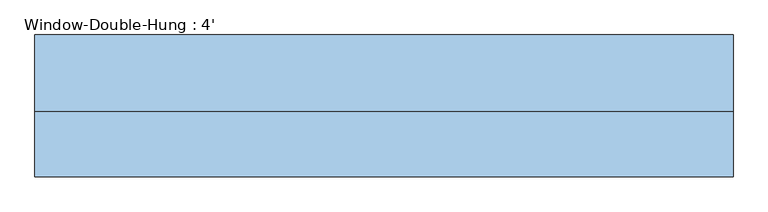
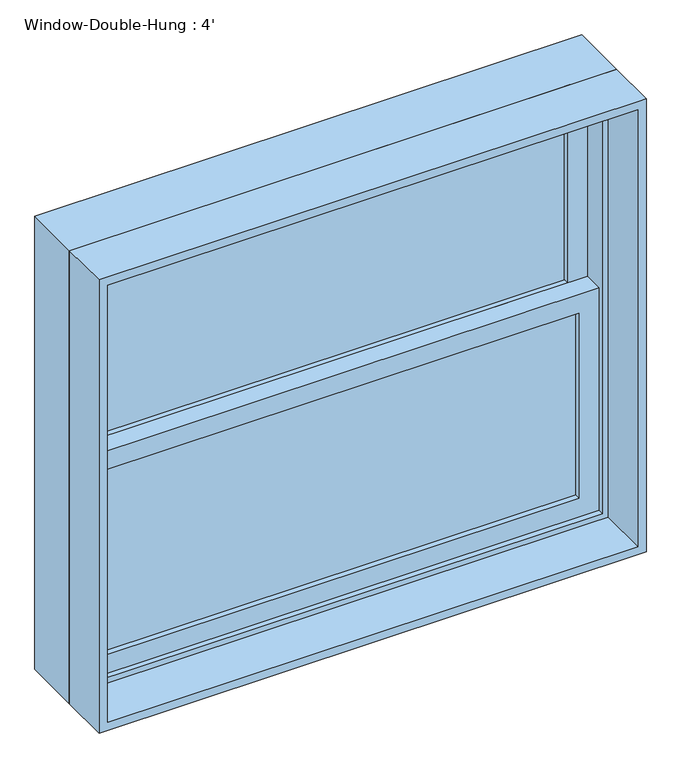
"""IFC4 building model written with IfcOpenShell, lengths in millimetres: window geometry, Window-Double-Hung : 4'."""

from ifc_helpers import new_model, si_unit, frame, origin, place, context, project, spatial, polyline, outline, extrude, source, transform, mapped, element, save


def window_double_hung_4_eadb0177(model_context):
    return source(origin(), model_context, "Body", "SweptSolid", [
        extrude(outline(polyline([(533.4, 44.45), (533.4, 38.1), (-533.4, 38.1), (-533.4, 44.45), (533.4, 44.45)])), frame((0.0, 0.0, 990.6), z_axis=(0.0, 0.0, 1.0), x_axis=(1.0, 0.0, 0.0)), (0.0, 0.0, 1.0), 434.975),
        extrude(outline(polyline([(-533.4, 31.75), (533.4, 31.75), (533.4, 25.4), (-533.4, 25.4), (-533.4, 31.75)])), frame((0.0, 0.0, 990.6), z_axis=(0.0, 0.0, 1.0), x_axis=(1.0, 0.0, 0.0)), (0.0, 0.0, 1.0), 434.975),
        extrude(outline(polyline([(533.4, 88.9), (533.4, 82.55), (-533.4, 82.55), (-533.4, 88.9), (533.4, 88.9)])), frame((0.0, 0.0, 1470.025), z_axis=(0.0, 0.0, 1.0), x_axis=(1.0, 0.0, 0.0)), (0.0, 0.0, 1.0), 434.975),
        extrude(outline(polyline([(-533.4, 76.2), (533.4, 76.2), (533.4, 69.85), (-533.4, 69.85), (-533.4, 76.2)])), frame((0.0, 0.0, 1470.025), z_axis=(0.0, 0.0, 1.0), x_axis=(1.0, 0.0, 0.0)), (0.0, 0.0, 1.0), 434.975),
        extrude(outline(polyline([(1470.025, -577.85), (946.15, -577.85), (946.15, 577.85), (1470.025, 577.85), (1470.025, -577.85)]), holes=[polyline([(1425.575, 533.4), (990.6, 533.4), (990.6, -533.4), (1425.575, -533.4), (1425.575, 533.4)])]), frame((0.0, 12.7, 0.0), z_axis=(0.0, 1.0, 0.0), x_axis=(0.0, 0.0, 1.0)), (0.0, 0.0, 1.0), 44.45),
        extrude(outline(polyline([(1949.45, -577.85), (1425.575, -577.85), (1425.575, 577.85), (1949.45, 577.85), (1949.45, -577.85)]), holes=[polyline([(1905.0, 533.4), (1470.025, 533.4), (1470.025, -533.4), (1905.0, -533.4), (1905.0, 533.4)])]), frame((0.0, 57.15, 0.0), z_axis=(0.0, 1.0, 0.0), x_axis=(0.0, 0.0, 1.0)), (0.0, 0.0, 1.0), 44.45),
        extrude(outline(polyline([(1981.2, -609.6), (914.4, -609.6), (914.4, 609.6), (1981.2, 609.6), (1981.2, -609.6)]), holes=[polyline([(1949.45, 577.85), (946.15, 577.85), (946.15, -577.85), (1949.45, -577.85), (1949.45, 577.85)])]), frame((0.0, 0.0, 0.0), z_axis=(0.0, 1.0, 0.0), x_axis=(0.0, 0.0, 1.0)), (0.0, 0.0, 1.0), 133.35),
        extrude(outline(polyline([(1981.2, 609.6), (1981.2, -609.6), (914.4, -609.6), (914.4, 609.6), (1981.2, 609.6)]), holes=[polyline([(1962.15, 590.55), (933.45, 590.55), (933.45, -590.55), (1962.15, -590.55), (1962.15, 590.55)])]), frame((0.0, -114.3, 0.0), z_axis=(0.0, 1.0, 0.0), x_axis=(0.0, 0.0, 1.0)), (0.0, 0.0, 1.0), 114.3),
    ])


if __name__ == "__main__":
    model = new_model("IFC4")
    model_context = context("Model", 3, world=origin())
    ifc_project = project(units=[si_unit("LENGTHUNIT", "METRE", prefix="MILLI")], contexts=[model_context])
    site = spatial("IfcSite", under=ifc_project)
    building = spatial("IfcBuilding", under=site)
    placement = place(None, origin())
    window_double_hung_4_shape = window_double_hung_4_eadb0177(model_context)
    element("IfcWindow", 1, ObjectType="Window-Double-Hung : 4'", at=placement, inside=building, context=model_context, shape_type="MappedRepresentation", body=[
        mapped(window_double_hung_4_shape, transform((0.0, 0.0, 0.0), x_axis=(1.0, 0.0, 0.0), y_axis=(0.0, 1.0, 0.0), z_axis=(0.0, 0.0, 1.0))),
    ])
    save(model, "model.ifc")

# Revit data of these elements
# Type "Window-Double-Hung : 4'"
#   Type Mark = "24"
#   Fire Rating = "0.5h"
#   Construction Type Id = "DG-DR"
#   Assembly Code = "B2020100"
#   Analytic Construction = "Double glazing - domestic"
#   Wall Thickness [instance default] = 0' - 6"
#   Window Inset [instance default] = 0' - 0"
#   Visual Light Transmittance = 0.81
#   Thermal Resistance (R) = 1.8146 (h·ft²·°F)/BTU
#   Solar Heat Gain Coefficient = 0.76
#   Muntin Width = 3' - 6"
#   Muntin Height = 1' - 5 1/8"
#   Interior Wall Closure [instance default] = 0' - 1 1/2"
#   Rough Width = 4' - 0 1/2"
#   Rough Height = 3' - 6 1/2"
#   Frame Extension [instance default] = 0' - 1 1/4"
#   Exterior Wall Closure [instance default] = 0' - 0 1/2"
#   Extension Jamb [instance default] = 0' - 1 1/2"
#   Heat Transfer Coefficient (U) = 0.5511 BTU/(h·ft²·°F)
#   Height = 3' - 6"
#   Width = 4' - 0"
#   Top Muntin Visibility = yes
#   Indicator Visibility [instance default] = yes
#   Extension Jamb Visibility [instance default] = yes
#   Interior Trim Visibility [instance default] = yes
#   Exterior Trim Visibility [instance default] = yes
#   Define Thermal Properties by = 1
#   Bottom Muntin Visibility = yes
#   Muntin Pattern = Muntin Pattern_2x2 : Muntin Pattern_2x2
#   Interior Trim Material = Wood - Stained
#   Interior Trim = Trim-Window-Interior-Flat : Picture Frame
#   Exterior Trim Material = Clad - White
#   Exterior Trim = Trim-Window-Exterior-Flat : with Sill
#   Glass Panel Material = Glass
#   Exterior Frame Material = Clad - White
#   Interior Frame Material = Wood - Stained
#   Wall Closure = (empty or 0)
# Element 1 (IfcWindow, "Window-Double-Hung : 4'")
#   Wall Thickness = 0' - 9"
#   Extension Jamb = 0' - 4 1/2"
#   Materials on its faces: "Wood - Stained", "Glass", "Clad - White"
# Materials
#   "Wood - Stained": class "Wood", colour RGB 224 178 126, transparency 0, Cost = 0
#   "Clad - White": class "Wood", colour RGB 242 242 238, transparency 0, Cost = 0
#   "Glass": class "Glass", colour RGB 0 128 192, transparency 0.75, Description = "Soda Lime Glass", Cost = 0
